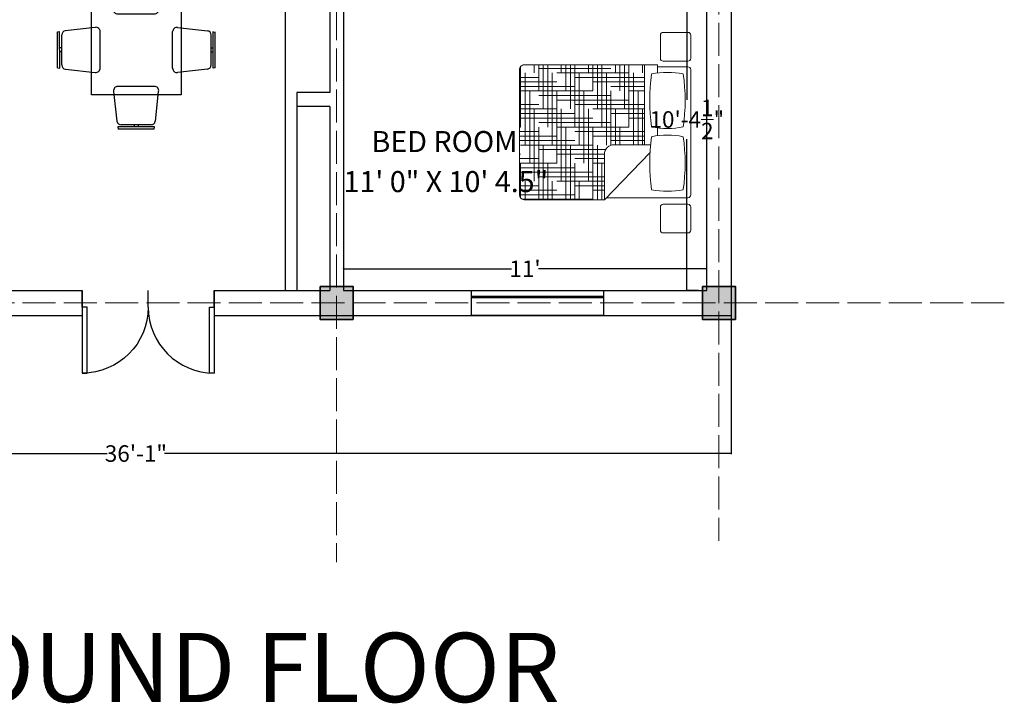
# Model space of a CAD drawing. Units: inches. Extents: x -113 to 5399, y -1393 to 3302.
# Tile 32 of 40: x 3405 to 3763, y 2439 to 2688. Entities that reach past the tile are written whole.
import ezdxf

# ---------------------------------------------------------------- set-up
doc = ezdxf.new("R2010")
doc.units = ezdxf.units.IN
doc.header["$MEASUREMENT"] = 0
doc.linetypes.add('ACAD_ISO02W100', pattern=[15, 12, -3])
for name, color, linetype, lineweight in [('A-ANNO-DIMS', 254, 'Continuous', 18), ('A-ANNO-TEXT', 7, 'Continuous', 25), ('A-AREA-IDEN', 4, 'Continuous', 18), ('A-COLS', 7, 'Continuous', 35), ('doors', 2, 'Continuous', 25), ('furniture', 131, 'Continuous', 18), ('GRIDS', 7, 'ACAD_ISO02W100', 13), ('walls', 1, 'Continuous', 25), ('windows', 3, 'Continuous', 25)]:
    doc.layers.add(name, color=color, linetype=linetype, lineweight=lineweight)
doc.layers.add('B-FURNITURE', color=22, linetype='Continuous')
doc.styles.get("Standard").update_dxf_attribs({"font": 'arial.ttf'})
doc.dimstyles.get("Standard").update_dxf_attribs({"dimtxt": 6, "dimasz": 0.18, "dimexe": 0.18, "dimexo": 0.0625, "dimgap": 0.09, "dimtad": 0, "dimtih": 1, "dimtoh": 1, "dimdec": 1, "dimzin": 0, "dimdsep": 46, "dimlunit": 4, "dimtxsty": 'Standard', "dimblk": 'ARCHTICK', "dimcen": 0.09, "dimadec": 0, "dimazin": 0, "dimtfac": 1, "dimtdec": 1, "dimtofl": 0, "dimtmove": 0, "dimatfit": 3, "dimfxl": 1, "dimtolj": 1, "dimtzin": 0, "dimarcsym": 0})

# ---------------------------------------------------------------- blocks, each defined once
blk = doc.blocks.new('*U2')
for p, q in [((0, 0), (0, -6)), ((24, 0), (24, -6))]:
    blk.add_line(p, q)
blk.add_lwpolyline([(0, 0), (0, 24), (1.75, 24), (1.75, 0)], close=True)
blk.add_arc((0, 0), 24, 0, 90)
blk = doc.blocks.new('*X4')
at = {"color": 0}
for p, q in [((4.359, 18.562), (4.359, 18.646)), ((4.5, 18), (4.5, 18.646)), ((4.547, 18.188), (4.547, 18.646)), ((4.594, 18.375), (4.594, 18.646)), ((4.641, 18.562), (4.641, 18.646)), ((4.687, 18.609), (5.437, 18.609)), ((4.781, 18), (4.781, 18.646)), ((4.828, 18.188), (4.828, 18.646)), ((4.875, 18.375), (4.875, 18.646)), ((4.922, 18.562), (4.922, 18.646)), ((5.062, 18), (5.062, 18.646)), ((5.109, 18.188), (5.109, 18.646)), ((5.156, 18.375), (5.156, 18.646)), ((5.203, 18.562), (5.203, 18.646)), ((5.344, 18), (5.344, 18.646)), ((5.391, 18.188), (5.391, 18.646)), ((5.437, 18.375), (5.437, 18.646)), ((5.484, 18.562), (5.484, 18.646)), ((5.625, 18), (5.625, 18.629)), ((4.34, 18.516), (5.062, 18.516)), ((4.453, 17.817), (4.453, 18.562)), ((4.5, 18.562), (5.25, 18.562)), ((4.734, 17.812), (4.734, 18.562)), ((5.016, 17.812), (5.016, 18.562)), ((5.297, 17.812), (5.297, 18.562)), ((5.437, 18.516), (5.637, 18.516)), ((5.578, 17.812), (5.578, 18.562)), ((5.625, 18.562), (5.637, 18.562)), ((4.34, 18.469), (4.875, 18.469)), ((4.34, 18.422), (4.687, 18.422)), ((5.062, 18.422), (5.637, 18.422)), ((5.25, 18.469), (5.637, 18.469)), ((4.34, 18.375), (4.5, 18.375)), ((4.406, 17.817), (4.406, 18.375)), ((4.687, 18.328), (5.437, 18.328)), ((4.687, 17.811), (4.687, 18.375)), ((4.875, 18.375), (5.625, 18.375)), ((4.969, 17.625), (4.969, 18.375)), ((5.25, 17.625), (5.25, 18.375)), ((5.531, 17.625), (5.531, 18.375)), ((4.34, 18.234), (5.062, 18.234)), ((4.5, 18.281), (5.25, 18.281)), ((5.437, 18.234), (5.637, 18.234)), ((5.625, 18.281), (5.637, 18.281)), ((4.34, 18.188), (4.875, 18.188)), ((4.34, 18.141), (4.687, 18.141)), ((4.359, 17.817), (4.359, 18.188)), ((4.641, 17.817), (4.641, 18.188)), ((4.922, 17.438), (4.922, 18.188)), ((5.062, 18.141), (5.637, 18.141)), ((5.203, 17.438), (5.203, 18.188)), ((5.25, 18.188), (5.637, 18.188)), ((5.484, 17.438), (5.484, 18.188)), ((4.34, 18.094), (4.5, 18.094)), ((4.5, 18), (5.25, 18)), ((4.594, 17.817), (4.594, 18)), ((4.687, 18.047), (5.437, 18.047)), ((4.875, 18.094), (5.625, 18.094)), ((4.875, 17.25), (4.875, 18)), ((5.156, 17.25), (5.156, 18)), ((5.437, 17.25), (5.437, 18)), ((5.625, 18), (5.637, 18)), ((4.34, 17.953), (5.062, 17.953)), ((4.34, 17.906), (4.875, 17.906)), ((5.25, 17.906), (5.637, 17.906)), ((5.437, 17.953), (5.637, 17.953)), ((4.34, 17.859), (4.687, 17.859)), ((4.828, 17.246), (4.828, 17.812)), ((4.875, 17.812), (5.625, 17.812)), ((5.062, 17.859), (5.637, 17.859)), ((5.109, 17.246), (5.109, 17.812)), ((5.391, 17.246), (5.391, 17.812)), ((4.742, 17.766), (5.437, 17.766)), ((4.755, 17.719), (5.25, 17.719)), ((5.625, 17.719), (5.637, 17.719)), ((4.755, 17.672), (5.062, 17.672)), ((4.755, 17.625), (4.875, 17.625)), ((4.781, 17.246), (4.781, 17.625)), ((5.062, 17.246), (5.062, 17.625)), ((5.25, 17.625), (5.637, 17.625)), ((5.344, 17.246), (5.344, 17.625)), ((5.437, 17.672), (5.637, 17.672)), ((5.625, 17.263), (5.625, 17.625)), ((4.755, 17.484), (5.437, 17.484)), ((4.875, 17.531), (5.625, 17.531)), ((5.062, 17.578), (5.637, 17.578)), ((4.755, 17.438), (5.25, 17.438)), ((4.755, 17.391), (5.062, 17.391)), ((5.016, 17.246), (5.016, 17.438)), ((5.297, 17.246), (5.297, 17.438)), ((5.437, 17.391), (5.637, 17.391)), ((5.578, 17.246), (5.578, 17.438)), ((5.625, 17.438), (5.637, 17.438)), ((4.755, 17.344), (4.875, 17.344)), ((5.062, 17.297), (5.637, 17.297)), ((5.25, 17.344), (5.637, 17.344)), ((4.875, 17.25), (5.608, 17.25)), ((4.969, 17.246), (4.969, 17.25)), ((5.25, 17.246), (5.25, 17.25)), ((5.531, 17.246), (5.531, 17.25))]:
    blk.add_line(p, q, dxfattribs=at)
blk = doc.blocks.new('MAT-P01')
for p, q in [((0.009, 0.846), (0.247, 0.846)), ((0.374, 0.846), (1.674, 0.846)), ((1.792, 0.846), (2.031, 0.846)), ((-0.021, 0.816), (-0.021, 0.56)), ((0.277, 0.816), (0.277, 0.56)), ((0.344, 0.816), (0.344, -0.032)), ((1.704, 0.816), (1.704, 0.5)), ((1.762, 0.816), (1.762, 0.56)), ((2.061, 0.816), (2.061, 0.56)), ((0.009, 0.53), (0.247, 0.53)), ((1.792, 0.53), (2.031, 0.53)), ((0.815, 0.423), (0.324, -0.051)), ((0.895, 0.429), (0.895, 0.049)), ((0.988, 0.5), (1.069, 0.5)), ((1.639, 0.5), (1.724, 0.5)), ((1.724, 0.5), (1.724, -0.884)), ((0.895, 0.364), (1.724, 0.364)), ((0.895, 0.364), (0.895, 0.049)), ((0.895, 0.364), (1.724, 0.364)), ((1.724, 0.364), (1.724, -0.884)), ((0.324, -0.051), (0.795, -0.051)), ((0.324, -0.051), (0.324, -0.884)), ((0.374, -0.934), (1.674, -0.934))]:
    blk.add_line(p, q)
for centre, radius, start, end in [((0.009, 0.816), 0.03, 90, 180), ((0.247, 0.816), 0.03, 0, 90), ((0.374, 0.816), 0.03, 90, 180), ((1.674, 0.816), 0.03, 0, 90), ((1.792, 0.816), 0.03, 90, 180), ((2.031, 0.816), 0.03, 0, 90), ((1.225, 0.603), 0.814, 168.373, 191.627), ((0.703, -1.144), 1.931, 81.8162, 98.1838), ((0.181, 0.603), 0.814, 348.373, 11.627), ((1.877, 0.603), 0.814, 168.373, 191.627), ((1.354, -1.144), 1.931, 81.8162, 98.1838), ((0.832, 0.603), 0.814, 348.373, 11.627), ((0.009, 0.56), 0.03, 180, 270), ((0.247, 0.56), 0.03, 270, 0), ((1.792, 0.56), 0.03, 180, 270), ((2.031, 0.56), 0.03, 270, 0), ((0.703, 2.35), 1.931, 261.8162, 278.1838), ((1.354, 2.35), 1.931, 261.8162, 278.1838), ((0.795, 0.049), 0.1, 270, 0), ((0.374, -0.884), 0.05, 180, 270), ((1.674, -0.884), 0.05, 270, 0)]:
    blk.add_arc(centre, radius, start, end)
at = {"rotation": 270}
blk.add_blockref('*X4', (-16.922, 4.704), dxfattribs=at)
blk = doc.blocks.new('A$C6ACA79D1')
at = {"layer": 'B-FURNITURE'}
for p, q in [((-0.503, 0.053), (-0.801, -0.244)), ((-0.483, 0.039), (-0.787, -0.264)), ((-0.503, 0.053), (-0.483, 0.039)), ((-0.429, 0), (-0.155, -0.22)), ((0.787, -0.259), (0.483, 0.044)), ((0.484, 0.043), (0.504, 0.058)), ((0.743, -0.249), (0.493, 0)), ((0.801, -0.239), (0.503, 0.059)), ((-0.493, -0.005), (-0.743, -0.254)), ((-0.601, -0.112), (-0.618, -0.095)), ((0.601, -0.107), (0.618, -0.09)), ((-0.635, -0.147), (-0.652, -0.13)), ((0.635, -0.142), (0.652, -0.124)), ((-0.786, -0.264), (-0.8, -0.244)), ((-0.148, -0.296), (-0.451, -0.599)), ((0.451, -0.594), (0.148, -0.291)), ((0.748, -0.313), (0.527, -0.588)), ((0.801, -0.239), (0.787, -0.259)), ((-0.148, -1.194), (-0.451, -0.891)), ((0.451, -0.896), (0.148, -1.199)), ((0.748, -1.177), (0.527, -0.902)), ((-0.503, -1.544), (-0.801, -1.246)), ((-0.786, -1.227), (-0.8, -1.247)), ((-0.483, -1.529), (-0.787, -1.226)), ((-0.493, -1.485), (-0.743, -1.236)), ((0.787, -1.231), (0.483, -1.535)), ((0.743, -1.241), (0.493, -1.49)), ((0.801, -1.251), (0.503, -1.549)), ((0.801, -1.251), (0.787, -1.231)), ((-0.635, -1.343), (-0.652, -1.361)), ((-0.601, -1.378), (-0.618, -1.395)), ((-0.429, -1.49), (-0.155, -1.27)), ((0.601, -1.383), (0.618, -1.4)), ((0.635, -1.349), (0.652, -1.366)), ((-0.503, -1.544), (-0.483, -1.529)), ((0.484, -1.534), (0.504, -1.548))]:
    blk.add_line(p, q, dxfattribs=at)
at = {"layer": 'B-FURNITURE', "ltscale": 300}
for p, q in [((0.155, -0.215), (0.429, 0.005)), ((-0.527, -0.593), (-0.748, -0.319)), ((-0.527, -0.897), (-0.748, -1.172)), ((0.155, -1.275), (0.429, -1.496))]:
    blk.add_line(p, q, dxfattribs=at)
blk.add_lwpolyline([(-0.742, -0.742), (0, 0), (0.742, -0.742), (0, -1.485)], close=True, dxfattribs=at)
at = {"layer": 'B-FURNITURE', "ltscale": 400}
for centre, start, end in [((-0.458, -0.04), 54.4069, 135), ((0.459, -0.036), 45, 125.5931), ((-0.706, -0.289), 135, 215.5931), ((0.707, -0.284), 324.4069, 45), ((-0.706, -1.201), 144.4069, 225), ((0.707, -1.206), 315, 35.5931), ((-0.458, -1.45), 225, 305.5931), ((0.459, -1.454), 234.4069, 315)]:
    blk.add_arc(centre, 0.0499, start, end, dxfattribs=at)
at = {"layer": 'B-FURNITURE', "ltscale": 300}
for centre, start, end in [((-0.184, -0.261), 315, 54.4069), ((0.184, -0.256), 125.5931, 225), ((-0.487, -0.564), 215.5931, 315), ((0.487, -0.559), 225, 324.4069), ((-0.487, -0.926), 45, 144.4069), ((0.487, -0.931), 35.5931, 135), ((-0.184, -1.229), 305.5931, 45), ((0.184, -1.234), 135, 234.4069)]:
    blk.add_arc(centre, 0.05, start, end, dxfattribs=at)
blk = doc.blocks.new('_ArchTick')
at = {"color": 0, "linetype": 'ByBlock', "const_width": 0.15}
blk.add_lwpolyline([(-0.5, -0.5), (0.5, 0.5)], dxfattribs=at)
blk = doc.blocks.new('*D129')
at = {"layer": 'A-ANNO-DIMS', "color": 0, "lineweight": -2, "transparency": 16777216}
for p, q in [((3230.55, 2580), (3230.55, 2529.62)), ((3663.55, 2580), (3663.55, 2529.62)), ((3230.55, 2529.8), (3436.65, 2529.8)), ((3663.55, 2529.8), (3457.44, 2529.8))]:
    blk.add_line(p, q, dxfattribs=at)
at = {"layer": 'Defpoints', "color": 0, "transparency": 16777216}
for p in [(3230.55, 2580.06), (3663.55, 2580.06), (3663.55, 2529.8)]:
    blk.add_point(p, dxfattribs=at)
at = {"layer": 'A-ANNO-DIMS', "color": 0, "lineweight": -2, "transparency": 16777216, "xscale": 0.18, "yscale": 0.18, "zscale": 0.18, "rotation": 180}
blk.add_blockref('_ArchTick', (3230.55, 2529.8), dxfattribs=at)
at = {"layer": 'A-ANNO-DIMS', "color": 0, "lineweight": -2, "transparency": 16777216, "xscale": 0.18, "yscale": 0.18, "zscale": 0.18}
blk.add_blockref('_ArchTick', (3663.55, 2529.8), dxfattribs=at)
at = {"layer": 'A-ANNO-DIMS', "color": 0, "transparency": 16777216, "insert": (3447.05, 2529.8), "char_height": 6, "attachment_point": 5}
blk.add_mtext('\\A1;36\'-1"', dxfattribs=at)
blk = doc.blocks.new('*D127')
at = {"layer": 'A-ANNO-DIMS', "color": 0, "lineweight": -2, "transparency": 16777216}
for p, q in [((3501.73, 2860.06), (3501.22, 2860.06)), ((3501.4, 2860.06), (3501.4, 2727.66)), ((3501.4, 2589.06), (3501.4, 2721.46)), ((3501.73, 2589.06), (3501.22, 2589.06))]:
    blk.add_line(p, q, dxfattribs=at)
at = {"layer": 'Defpoints', "color": 0, "transparency": 16777216}
for p in [(3501.8, 2860.06), (3501.4, 2589.06), (3501.8, 2589.06)]:
    blk.add_point(p, dxfattribs=at)
at = {"layer": 'A-ANNO-DIMS', "color": 0, "lineweight": -2, "transparency": 16777216, "xscale": 0.18, "yscale": 0.18, "zscale": 0.18}
for p, rotation in [((3501.4, 2860.06), 90), ((3501.4, 2589.06), 270)]:
    blk.add_blockref('_ArchTick', p, dxfattribs=dict(at, rotation=rotation))
at = {"layer": 'A-ANNO-DIMS', "color": 0, "transparency": 16777216, "insert": (3501.4, 2724.56), "char_height": 6, "attachment_point": 5}
blk.add_mtext('\\A1;22\'-7"', dxfattribs=at)
blk = doc.blocks.new('*D140')
at = {"layer": 'A-ANNO-DIMS', "color": 0, "lineweight": -2, "transparency": 16777216}
for p, q in [((3522.55, 2597.07), (3522.55, 2597.19)), ((3522.55, 2597.01), (3583.65, 2597.01)), ((3654.55, 2597.01), (3593.45, 2597.01)), ((3654.55, 2597.07), (3654.55, 2597.19))]:
    blk.add_line(p, q, dxfattribs=at)
at = {"layer": 'Defpoints', "color": 0, "transparency": 16777216}
for p in [(3522.55, 2597.01), (3522.55, 2597.01), (3654.55, 2597.01)]:
    blk.add_point(p, dxfattribs=at)
at = {"layer": 'A-ANNO-DIMS', "color": 0, "lineweight": -2, "transparency": 16777216, "xscale": 0.18, "yscale": 0.18, "zscale": 0.18, "rotation": 180}
blk.add_blockref('_ArchTick', (3522.55, 2597.01), dxfattribs=at)
at = {"layer": 'A-ANNO-DIMS', "color": 0, "lineweight": -2, "transparency": 16777216, "xscale": 0.18, "yscale": 0.18, "zscale": 0.18}
blk.add_blockref('_ArchTick', (3654.55, 2597.01), dxfattribs=at)
at = {"layer": 'A-ANNO-DIMS', "color": 0, "transparency": 16777216, "insert": (3588.55, 2597.01), "char_height": 6, "attachment_point": 5}
blk.add_mtext("\\A1;11'", dxfattribs=at)
blk = doc.blocks.new('*D141')
at = {"layer": 'A-ANNO-DIMS', "color": 0, "lineweight": -2, "transparency": 16777216}
for p, q in [((3651.65, 2713.56), (3647.23, 2713.56)), ((3647.41, 2713.56), (3647.41, 2658.47)), ((3647.41, 2589.06), (3647.41, 2644.14)), ((3651.65, 2589.06), (3647.23, 2589.06))]:
    blk.add_line(p, q, dxfattribs=at)
at = {"layer": 'Defpoints', "color": 0, "transparency": 16777216}
for p in [(3651.72, 2713.56), (3647.41, 2589.06), (3651.72, 2589.06)]:
    blk.add_point(p, dxfattribs=at)
at = {"layer": 'A-ANNO-DIMS', "color": 0, "lineweight": -2, "transparency": 16777216, "xscale": 0.18, "yscale": 0.18, "zscale": 0.18}
for p, rotation in [((3647.41, 2713.56), 90), ((3647.41, 2589.06), 270)]:
    blk.add_blockref('_ArchTick', p, dxfattribs=dict(at, rotation=rotation))
at = {"layer": 'A-ANNO-DIMS', "color": 0, "transparency": 16777216, "insert": (3647.41, 2651.31), "char_height": 6, "attachment_point": 5}
blk.add_mtext('\\A1;10\'-4{\\H1x;\\S1/2;}"', dxfattribs=at)
blk = doc.blocks.new('WIN-PLAN-48IN')
h = blk.add_hatch(color=256)
h.dxf.hatch_style = 1
h.paths.add_polyline_path([(48, 2.5), (0, 2.5), (0, 2), (48, 2)])
for p, q in [((0, 9), (48, 9)), ((0, 0), (0, 9)), ((48, 9), (48, 0)), ((48, 2.5), (0, 2.5)), ((48, 2), (0, 2)), ((48, 0), (0, 0))]:
    blk.add_line(p, q)
blk = doc.blocks.new('COLUMN-12IN-SQUARE')
h = blk.add_hatch(color=256)
h.dxf.hatch_style = 1
h.paths.add_polyline_path([(6, 6), (-6, 6), (-6, -6), (6, -6)])
blk.add_lwpolyline([(-6, 6), (6, 6), (6, -6), (-6, -6)], close=True)

msp = doc.modelspace()

# ---------------------------------------------------------------- linework, layer by layer
at = {"layer": 'GRIDS'}
for p, q in [((3659.05, 3271.46), (3659.05, 2498.02)), ((3520.05, 3262.17), (3520.05, 2490.34)), ((3762.86, 2584.56), (3104.61, 2584.56))]:
    msp.add_line(p, q, dxfattribs=at)
at = {"layer": 'walls'}
for p, q in [((3663.55, 3230.06), (3663.55, 2580.06)), ((3517.55, 2735.56), (3517.55, 2661.06)), ((3522.55, 2735.56), (3522.55, 2589.06)), ((3654.55, 2713.56), (3654.55, 2589.06)), ((3517.55, 2661.06), (3505.55, 2661.06)), ((3505.55, 2661.06), (3505.55, 2656.06)), ((3517.55, 2656.06), (3505.55, 2656.06)), ((3505.55, 2656.06), (3505.55, 2589.06)), ((3517.55, 2656.06), (3517.55, 2589.06)), ((3385.55, 2589.06), (3427.55, 2589.06)), ((3427.55, 2589.06), (3427.55, 2580.06)), ((3475.55, 2589.06), (3517.55, 2589.06)), ((3475.55, 2589.06), (3475.55, 2580.06)), ((3522.55, 2589.06), (3654.55, 2589.06)), ((3230.55, 2580.06), (3427.55, 2580.06)), ((3475.55, 2580.06), (3569.05, 2580.06)), ((3522.55, 2580.06), (3663.55, 2580.06))]:
    msp.add_line(p, q, dxfattribs=at)

# ---------------------------------------------------------------- block references
at = {"layer": 'A-COLS'}
for p in [(3520.05, 2584.56), (3659.05, 2584.56)]:
    msp.add_blockref('COLUMN-12IN-SQUARE', p, dxfattribs=at)
at = {"layer": 'doors', "xscale": -1, "rotation": 180}
msp.add_blockref('*U2', (3427.55, 2583.06), dxfattribs=at)
at = {"layer": 'doors', "rotation": 180}
msp.add_blockref('*U2', (3475.55, 2583.06), dxfattribs=at)
at = {"layer": 'furniture'}
for name, p, xscale, yscale, zscale, rotation in [('A$C6ACA79D1', (3463.54, 2692.92), 31.0665876167328, 31.0665876167328, 31.0665876167328, 314.9999999999397), ('MAT-P01', (3619.22, 2610.79), -35.02364872074636, 35.02364872074636, 35.02364872074636, 270)]:
    msp.add_blockref(name, p, dxfattribs=dict(at, xscale=xscale, yscale=yscale, zscale=zscale, rotation=rotation))
at = {"layer": 'windows', "rotation": 180}
msp.add_blockref('WIN-PLAN-48IN', (3617.05, 2589.06), dxfattribs=at)

# ---------------------------------------------------------------- texts
at = {"layer": 'A-ANNO-TEXT'}
msp.add_text('GROUND FLOOR', height=25.17, dxfattribs=at).set_placement((3339.05, 2439.4))
at = {"layer": 'A-AREA-IDEN'}
for s, height, p in [('BED ROOM', 7.647, (3532.73, 2639.46)), ('11\' 0" X 10\' 4.5"', 7.6473, (3522.55, 2624.89))]:
    msp.add_text(s, height=height, dxfattribs=at).set_placement(p)

# ---------------------------------------------------------------- dimensions: what is measured, and where the dimension line sits
at = {"layer": 'A-ANNO-DIMS'}
for base, p1, p2, picture, middle in [((3501.4, 2589.06), (3501.8, 2860.06), (3501.8, 2589.06), '*D127', (3501.4, 2724.56)), ((3647.41, 2589.06), (3651.72, 2713.56), (3651.72, 2589.06), '*D141', (3647.41, 2651.31))]:
    dim = msp.add_linear_dim(base=base, p1=p1, p2=p2, angle=90, dimstyle='Standard', override={"dimclrd": 0, "dimclre": 0, "dimclrt": 0}, dxfattribs=at)
    dim.commit()
    dim.dimension.update_dxf_attribs({"geometry": picture, "text_midpoint": middle})
for base, p1, p2, picture, middle in [((3522.55, 2597.01), (3654.55, 2597.01), (3522.55, 2597.01), '*D140', (3588.55, 2597.01)), ((3663.55, 2529.8), (3230.55, 2580.06), (3663.55, 2580.06), '*D129', (3447.05, 2529.8))]:
    dim = msp.add_linear_dim(base=base, p1=p1, p2=p2, dimstyle='Standard', override={"dimclrd": 0, "dimclre": 0, "dimclrt": 0}, dxfattribs=at)
    dim.commit()
    dim.dimension.update_dxf_attribs({"geometry": picture, "text_midpoint": middle})

doc.saveas('drawing.dxf')
